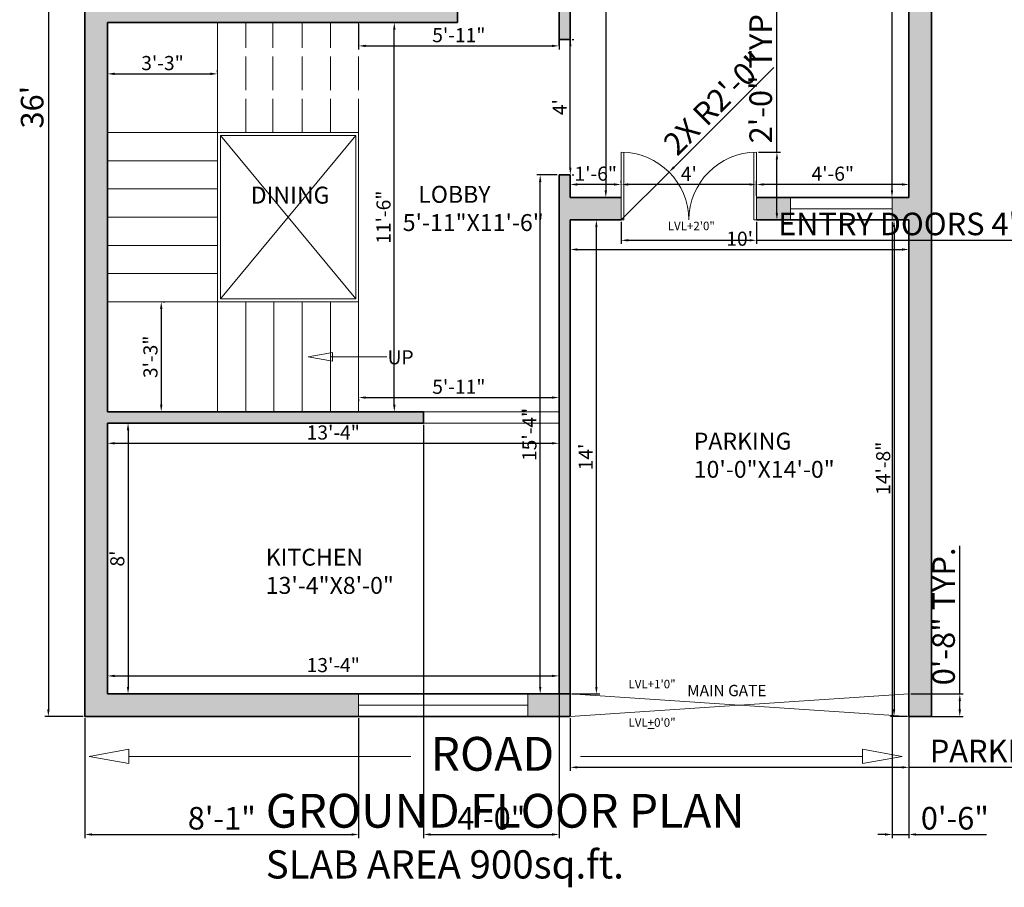
# Model space of a CAD drawing. Units: inches. Extents: x 3259 to 4981, y 1402 to 2026.
# Tile 8 of 11: x 4265 to 4614, y 1415 to 1722. Entities that reach past the tile are written whole.
import ezdxf

# ---------------------------------------------------------------- set-up
doc = ezdxf.new("R2010")
doc.units = ezdxf.units.IN
doc.linetypes.add('ACAD_ISO02W100', pattern=[15, 12, -3])
for name, color, linetype, lineweight in [('A-ANNO-DIMS', 2, 'Continuous', 13), ('A-ANNO-SYMB', 7, 'Continuous', 13), ('A-ANNO-TEXT', 7, 'Continuous', 18), ('A-ANNO-TITL', 7, 'Continuous', 25), ('A-AREA-IDEN', 7, 'Continuous', 18), ('A-DOOR', 3, 'Continuous', 18), ('A-FLOR-STRS', 7, 'Continuous', 18), ('A-FLOR-STRS-OVHD', 8, 'ACAD_ISO02W100', 13), ('A-FURN', 8, 'Continuous', 13), ('A-GLAZ', 4, 'Continuous', 18), ('A-WALL', 7, 'Continuous', 35), ('A-WALL-PATT', 252, 'Continuous', 13)]:
    doc.layers.add(name, color=color, linetype=linetype, lineweight=lineweight)
doc.styles.get("Standard").update_dxf_attribs({"font": 'arial.ttf'})
doc.dimstyles.new('ISO-25', dxfattribs={"dimtxt": 8, "dimasz": 2.5, "dimexe": 1.25, "dimexo": 0.625, "dimtad": 1, "dimdec": 1, "dimlunit": 3, "dimtxsty": 'Standard', "dimcen": 2.5, "dimclrd": 4, "dimclre": 4, "dimclrt": 1, "dimadec": 0, "dimazin": 0, "dimtfac": 1, "dimtdec": 1, "dimtmove": 0, "dimatfit": 3, "dimfxl": 1, "dimarcsym": 0})

# ---------------------------------------------------------------- blocks, each defined once
blk = doc.blocks.new('*D84')
at = {"layer": 'A-ANNO-DIMS', "color": 0, "lineweight": -2, "transparency": 16777216}
for p, q in [((4287.71, 1907.12), (4274.14, 1907.12)), ((4275.39, 1904.62), (4275.39, 1477.62)), ((4287.71, 1475.12), (4274.14, 1475.12))]:
    blk.add_line(p, q, dxfattribs=at)
at = {"layer": 'A-ANNO-DIMS', "color": 0, "transparency": 16777216}
for points in [[(4274.97, 1904.62), (4275.81, 1904.62), (4275.39, 1907.12)], [(4274.97, 1477.62), (4275.81, 1477.62), (4275.39, 1475.12)]]:
    blk.add_solid(points, dxfattribs=at)
at = {"layer": 'Defpoints', "color": 0, "transparency": 16777216}
for p in [(4288.33, 1907.12), (4275.39, 1475.12), (4288.33, 1475.12)]:
    blk.add_point(p, dxfattribs=at)
at = {"layer": 'A-ANNO-DIMS', "color": 0, "transparency": 16777216, "insert": (4270.68, 1691.12), "char_height": 8, "attachment_point": 5, "rotation": 90}
blk.add_mtext("36'", dxfattribs=at)
blk = doc.blocks.new('*D80')
at = {"layer": 'A-ANNO-DIMS', "color": 0, "lineweight": -2, "transparency": 16777216}
for p, q in [((4460.96, 1847.12), (4474.15, 1847.12)), ((4472.9, 1844.62), (4472.9, 1661.62)), ((4460.96, 1659.12), (4474.15, 1659.12))]:
    blk.add_line(p, q, dxfattribs=at)
at = {"layer": 'A-ANNO-DIMS', "color": 0, "transparency": 16777216}
for points in [[(4472.49, 1844.62), (4473.32, 1844.62), (4472.9, 1847.12)], [(4472.49, 1661.62), (4473.32, 1661.62), (4472.9, 1659.12)]]:
    blk.add_solid(points, dxfattribs=at)
at = {"layer": 'Defpoints', "color": 0, "transparency": 16777216}
for p in [(4460.33, 1847.12), (4460.33, 1659.12), (4472.9, 1659.12)]:
    blk.add_point(p, dxfattribs=at)
at = {"layer": 'A-ANNO-DIMS', "color": 0, "transparency": 16777216, "insert": (4469.73, 1753.12), "char_height": 5, "attachment_point": 5, "rotation": 90}
blk.add_mtext('15\'-8"', dxfattribs=at)
blk = doc.blocks.new('*D81')
at = {"layer": 'A-ANNO-DIMS', "color": 0, "lineweight": -2, "transparency": 16777216}
for p, q in [((4385.33, 1587.56), (4385.33, 1586.93)), ((4387.83, 1588.18), (4453.83, 1588.18)), ((4456.33, 1588.81), (4456.33, 1589.43))]:
    blk.add_line(p, q, dxfattribs=at)
at = {"layer": 'A-ANNO-DIMS', "color": 0, "transparency": 16777216}
for points in [[(4387.83, 1588.6), (4387.83, 1587.76), (4385.33, 1588.18)], [(4453.83, 1588.6), (4453.83, 1587.76), (4456.33, 1588.18)]]:
    blk.add_solid(points, dxfattribs=at)
at = {"layer": 'Defpoints', "color": 0, "transparency": 16777216}
for p in [(4385.33, 1588.18), (4456.33, 1588.18), (4456.33, 1588.18)]:
    blk.add_point(p, dxfattribs=at)
at = {"layer": 'A-ANNO-DIMS', "color": 0, "transparency": 16777216, "insert": (4420.83, 1591.36), "char_height": 5, "attachment_point": 5}
blk.add_mtext('5\'-11"', dxfattribs=at)
blk = doc.blocks.new('*D82')
at = {"layer": 'A-ANNO-DIMS', "color": 0, "lineweight": -2, "transparency": 16777216}
for p, q in [((4396.19, 1721.12), (4399.22, 1721.12)), ((4397.97, 1585.62), (4397.97, 1718.62)), ((4393.89, 1583.12), (4399.22, 1583.12))]:
    blk.add_line(p, q, dxfattribs=at)
at = {"layer": 'A-ANNO-DIMS', "color": 0, "transparency": 16777216}
for points in [[(4397.55, 1718.62), (4398.39, 1718.62), (4397.97, 1721.12)], [(4397.55, 1585.62), (4398.39, 1585.62), (4397.97, 1583.12)]]:
    blk.add_solid(points, dxfattribs=at)
at = {"layer": 'Defpoints', "color": 0, "transparency": 16777216}
for p in [(4395.56, 1721.12), (4397.97, 1721.12), (4393.26, 1583.12)]:
    blk.add_point(p, dxfattribs=at)
at = {"layer": 'A-ANNO-DIMS', "color": 0, "transparency": 16777216, "insert": (4394.79, 1652.12), "char_height": 5, "attachment_point": 5, "rotation": 90}
blk.add_mtext('11\'-6"', dxfattribs=at)
blk = doc.blocks.new('*D74')
at = {"layer": 'A-ANNO-DIMS', "color": 0, "lineweight": -2, "transparency": 16777216}
for p, q in [((4296.33, 1703.55), (4296.33, 1704.17)), ((4298.83, 1702.92), (4332.83, 1702.92)), ((4335.33, 1703.55), (4335.33, 1704.17))]:
    blk.add_line(p, q, dxfattribs=at)
at = {"layer": 'A-ANNO-DIMS', "color": 0, "transparency": 16777216}
for points in [[(4298.83, 1703.34), (4298.83, 1702.51), (4296.33, 1702.92)], [(4332.83, 1703.34), (4332.83, 1702.51), (4335.33, 1702.92)]]:
    blk.add_solid(points, dxfattribs=at)
at = {"layer": 'Defpoints', "color": 0, "transparency": 16777216}
for p in [(4296.33, 1702.92), (4335.33, 1702.92), (4335.33, 1702.92)]:
    blk.add_point(p, dxfattribs=at)
at = {"layer": 'A-ANNO-DIMS', "color": 0, "transparency": 16777216, "insert": (4315.83, 1706.1), "char_height": 5, "attachment_point": 5}
blk.add_mtext('3\'-3"', dxfattribs=at)
blk = doc.blocks.new('*D75')
at = {"layer": 'A-ANNO-DIMS', "color": 0, "lineweight": -2, "transparency": 16777216}
for p, q in [((4315.38, 1619.62), (4315.38, 1585.62)), ((4316.01, 1622.12), (4316.63, 1622.12)), ((4316.01, 1583.12), (4316.63, 1583.12))]:
    blk.add_line(p, q, dxfattribs=at)
at = {"layer": 'A-ANNO-DIMS', "color": 0, "transparency": 16777216}
for points in [[(4314.97, 1619.62), (4315.8, 1619.62), (4315.38, 1622.12)], [(4314.97, 1585.62), (4315.8, 1585.62), (4315.38, 1583.12)]]:
    blk.add_solid(points, dxfattribs=at)
at = {"layer": 'Defpoints', "color": 0, "transparency": 16777216}
for p in [(4315.38, 1622.12), (4315.38, 1583.12), (4315.38, 1583.12)]:
    blk.add_point(p, dxfattribs=at)
at = {"layer": 'A-ANNO-DIMS', "color": 0, "transparency": 16777216, "insert": (4312.2, 1602.62), "char_height": 5, "attachment_point": 5, "rotation": 90}
blk.add_mtext('3\'-3"', dxfattribs=at)
blk = doc.blocks.new('*D76')
at = {"layer": 'A-ANNO-DIMS', "color": 0, "lineweight": -2, "transparency": 16777216}
for p, q in [((4296.33, 1578.49), (4296.33, 1570.72)), ((4456.33, 1578.49), (4456.33, 1570.72)), ((4298.83, 1571.97), (4453.83, 1571.97))]:
    blk.add_line(p, q, dxfattribs=at)
at = {"layer": 'A-ANNO-DIMS', "color": 0, "transparency": 16777216}
for points in [[(4298.83, 1572.39), (4298.83, 1571.56), (4296.33, 1571.97)], [(4453.83, 1572.39), (4453.83, 1571.56), (4456.33, 1571.97)]]:
    blk.add_solid(points, dxfattribs=at)
at = {"layer": 'Defpoints', "color": 0, "transparency": 16777216}
for p in [(4296.33, 1579.12), (4456.33, 1579.12), (4456.33, 1571.97)]:
    blk.add_point(p, dxfattribs=at)
at = {"layer": 'A-ANNO-DIMS', "color": 0, "transparency": 16777216, "insert": (4376.33, 1575.15), "char_height": 5, "attachment_point": 5}
blk.add_mtext('13\'-4"', dxfattribs=at)
blk = doc.blocks.new('*D77')
at = {"layer": 'A-ANNO-DIMS', "color": 0, "lineweight": -2, "transparency": 16777216}
for p, q in [((4296.96, 1579.12), (4304.87, 1579.12)), ((4303.62, 1576.62), (4303.62, 1485.62)), ((4296.96, 1483.12), (4304.87, 1483.12))]:
    blk.add_line(p, q, dxfattribs=at)
at = {"layer": 'A-ANNO-DIMS', "color": 0, "transparency": 16777216}
for points in [[(4303.21, 1576.62), (4304.04, 1576.62), (4303.62, 1579.12)], [(4303.21, 1485.62), (4304.04, 1485.62), (4303.62, 1483.12)]]:
    blk.add_solid(points, dxfattribs=at)
at = {"layer": 'Defpoints', "color": 0, "transparency": 16777216}
for p in [(4296.33, 1579.12), (4296.33, 1483.12), (4303.62, 1483.12)]:
    blk.add_point(p, dxfattribs=at)
at = {"layer": 'A-ANNO-DIMS', "color": 0, "transparency": 16777216, "insert": (4300.45, 1531.12), "char_height": 5, "attachment_point": 5, "rotation": 90}
blk.add_mtext("8'", dxfattribs=at)
blk = doc.blocks.new('*D78')
at = {"layer": 'A-ANNO-DIMS', "color": 0, "lineweight": -2, "transparency": 16777216}
for p, q in [((4460.96, 1651.12), (4470.82, 1651.12)), ((4469.57, 1485.62), (4469.57, 1648.62)), ((4460.96, 1483.12), (4470.82, 1483.12))]:
    blk.add_line(p, q, dxfattribs=at)
at = {"layer": 'A-ANNO-DIMS', "color": 0, "transparency": 16777216}
for points in [[(4469.16, 1648.62), (4469.99, 1648.62), (4469.57, 1651.12)], [(4469.16, 1485.62), (4469.99, 1485.62), (4469.57, 1483.12)]]:
    blk.add_solid(points, dxfattribs=at)
at = {"layer": 'Defpoints', "color": 0, "transparency": 16777216}
for p in [(4460.33, 1651.12), (4469.57, 1651.12), (4460.33, 1483.12)]:
    blk.add_point(p, dxfattribs=at)
at = {"layer": 'A-ANNO-DIMS', "color": 0, "transparency": 16777216, "insert": (4466.44, 1567.12), "char_height": 5, "attachment_point": 5, "rotation": 90}
blk.add_mtext("14'", dxfattribs=at)
blk = doc.blocks.new('*D64')
at = {"layer": 'A-ANNO-DIMS', "color": 0, "lineweight": -2, "transparency": 16777216}
for p, q in [((4460.33, 1650.49), (4460.33, 1639.41)), ((4580.33, 1650.49), (4580.33, 1639.41)), ((4462.83, 1640.66), (4577.83, 1640.66))]:
    blk.add_line(p, q, dxfattribs=at)
at = {"layer": 'A-ANNO-DIMS', "color": 0, "transparency": 16777216}
for points in [[(4462.83, 1641.08), (4462.83, 1640.25), (4460.33, 1640.66)], [(4577.83, 1641.08), (4577.83, 1640.25), (4580.33, 1640.66)]]:
    blk.add_solid(points, dxfattribs=at)
at = {"layer": 'Defpoints', "color": 0, "transparency": 16777216}
for p in [(4460.33, 1651.12), (4580.33, 1651.12), (4580.33, 1640.66)]:
    blk.add_point(p, dxfattribs=at)
at = {"layer": 'A-ANNO-DIMS', "color": 0, "transparency": 16777216, "insert": (4520.33, 1643.84), "char_height": 5, "attachment_point": 5}
blk.add_mtext("10'", dxfattribs=at)
blk = doc.blocks.new('*D107')
at = {"layer": 'A-ANNO-DIMS', "color": 0, "lineweight": -2, "transparency": 16777216}
for p, q in [((4296.33, 1483.74), (4296.33, 1490.78)), ((4456.33, 1483.74), (4456.33, 1490.78)), ((4298.83, 1489.53), (4453.83, 1489.53))]:
    blk.add_line(p, q, dxfattribs=at)
at = {"layer": 'A-ANNO-DIMS', "color": 0, "transparency": 16777216}
for points in [[(4298.83, 1489.94), (4298.83, 1489.11), (4296.33, 1489.53)], [(4453.83, 1489.94), (4453.83, 1489.11), (4456.33, 1489.53)]]:
    blk.add_solid(points, dxfattribs=at)
at = {"layer": 'Defpoints', "color": 0, "transparency": 16777216}
for p in [(4456.33, 1489.53), (4296.33, 1483.12), (4456.33, 1483.12)]:
    blk.add_point(p, dxfattribs=at)
at = {"layer": 'A-ANNO-DIMS', "color": 0, "transparency": 16777216, "insert": (4376.33, 1492.71), "char_height": 5, "attachment_point": 5}
blk.add_mtext('13\'-4"', dxfattribs=at)
blk = doc.blocks.new('*D108')
at = {"layer": 'A-ANNO-DIMS', "color": 0, "lineweight": -2, "transparency": 16777216}
for p, q in [((4455.71, 1667.12), (4448.41, 1667.12)), ((4449.66, 1485.62), (4449.66, 1664.62)), ((4455.71, 1483.12), (4448.41, 1483.12))]:
    blk.add_line(p, q, dxfattribs=at)
at = {"layer": 'A-ANNO-DIMS', "color": 0, "transparency": 16777216}
for points in [[(4449.24, 1664.62), (4450.08, 1664.62), (4449.66, 1667.12)], [(4449.24, 1485.62), (4450.08, 1485.62), (4449.66, 1483.12)]]:
    blk.add_solid(points, dxfattribs=at)
at = {"layer": 'Defpoints', "color": 0, "transparency": 16777216}
for p in [(4449.66, 1667.12), (4456.33, 1667.12), (4456.33, 1483.12)]:
    blk.add_point(p, dxfattribs=at)
at = {"layer": 'A-ANNO-DIMS', "color": 0, "transparency": 16777216, "insert": (4446.48, 1575.12), "char_height": 5, "attachment_point": 5, "rotation": 90}
blk.add_mtext('15\'-4"', dxfattribs=at)
blk = doc.blocks.new('*D115')
at = {"layer": 'A-ANNO-DIMS', "color": 0, "lineweight": -2, "transparency": 16777216}
for p, q in [((4579.71, 1851.12), (4573.06, 1851.12)), ((4574.31, 1848.62), (4574.31, 1661.62)), ((4579.71, 1659.12), (4573.06, 1659.12))]:
    blk.add_line(p, q, dxfattribs=at)
at = {"layer": 'A-ANNO-DIMS', "color": 0, "transparency": 16777216}
for points in [[(4573.9, 1848.62), (4574.73, 1848.62), (4574.31, 1851.12)], [(4573.9, 1661.62), (4574.73, 1661.62), (4574.31, 1659.12)]]:
    blk.add_solid(points, dxfattribs=at)
at = {"layer": 'Defpoints', "color": 0, "transparency": 16777216}
for p in [(4580.33, 1851.12), (4574.31, 1659.12), (4580.33, 1659.12)]:
    blk.add_point(p, dxfattribs=at)
at = {"layer": 'A-ANNO-DIMS', "color": 0, "transparency": 16777216, "insert": (4571.13, 1755.12), "char_height": 5, "attachment_point": 5, "rotation": 90}
blk.add_mtext("16'", dxfattribs=at)
blk = doc.blocks.new('*D116')
at = {"layer": 'A-ANNO-DIMS', "color": 0, "lineweight": -2, "transparency": 16777216}
for p, q in [((4526.33, 1659.74), (4526.33, 1664.96)), ((4580.33, 1659.74), (4580.33, 1664.96)), ((4577.83, 1663.71), (4528.83, 1663.71))]:
    blk.add_line(p, q, dxfattribs=at)
at = {"layer": 'A-ANNO-DIMS', "color": 0, "transparency": 16777216}
for points in [[(4528.83, 1664.13), (4528.83, 1663.29), (4526.33, 1663.71)], [(4577.83, 1664.13), (4577.83, 1663.29), (4580.33, 1663.71)]]:
    blk.add_solid(points, dxfattribs=at)
at = {"layer": 'Defpoints', "color": 0, "transparency": 16777216}
for p in [(4526.33, 1663.71), (4526.33, 1659.12), (4580.33, 1659.12)]:
    blk.add_point(p, dxfattribs=at)
at = {"layer": 'A-ANNO-DIMS', "color": 0, "transparency": 16777216, "insert": (4553.33, 1666.89), "char_height": 5, "attachment_point": 5}
blk.add_mtext('4\'-6"', dxfattribs=at)
blk = doc.blocks.new('*D117')
at = {"layer": 'A-ANNO-DIMS', "color": 0, "lineweight": -2, "transparency": 16777216}
for p, q in [((4478.33, 1664.34), (4478.33, 1664.96)), ((4526.33, 1659.74), (4526.33, 1664.96)), ((4523.83, 1663.71), (4480.83, 1663.71))]:
    blk.add_line(p, q, dxfattribs=at)
at = {"layer": 'A-ANNO-DIMS', "color": 0, "transparency": 16777216}
for points in [[(4480.83, 1664.13), (4480.83, 1663.29), (4478.33, 1663.71)], [(4523.83, 1664.13), (4523.83, 1663.29), (4526.33, 1663.71)]]:
    blk.add_solid(points, dxfattribs=at)
at = {"layer": 'Defpoints', "color": 0, "transparency": 16777216}
for p in [(4478.33, 1663.71), (4478.33, 1663.71), (4526.33, 1659.12)]:
    blk.add_point(p, dxfattribs=at)
at = {"layer": 'A-ANNO-DIMS', "color": 0, "transparency": 16777216, "insert": (4502.33, 1666.84), "char_height": 5, "attachment_point": 5}
blk.add_mtext("4'", dxfattribs=at)
blk = doc.blocks.new('*D118')
at = {"layer": 'A-ANNO-DIMS', "color": 0, "lineweight": -2, "transparency": 16777216}
for p, q in [((4460.33, 1663.74), (4460.33, 1664.96)), ((4478.33, 1664.34), (4478.33, 1664.96)), ((4475.83, 1663.71), (4462.83, 1663.71))]:
    blk.add_line(p, q, dxfattribs=at)
at = {"layer": 'A-ANNO-DIMS', "color": 0, "transparency": 16777216}
for points in [[(4462.83, 1664.13), (4462.83, 1663.29), (4460.33, 1663.71)], [(4475.83, 1664.13), (4475.83, 1663.29), (4478.33, 1663.71)]]:
    blk.add_solid(points, dxfattribs=at)
at = {"layer": 'Defpoints', "color": 0, "transparency": 16777216}
for p in [(4460.33, 1663.71), (4460.33, 1663.12), (4478.33, 1663.71)]:
    blk.add_point(p, dxfattribs=at)
at = {"layer": 'A-ANNO-DIMS', "color": 0, "transparency": 16777216, "insert": (4469.33, 1666.89), "char_height": 5, "attachment_point": 5}
blk.add_mtext('1\'-6"', dxfattribs=at)
blk = doc.blocks.new('*D119')
at = {"layer": 'A-ANNO-DIMS', "color": 0, "lineweight": -2, "transparency": 16777216}
for p, q in [((4385.33, 1720.49), (4385.33, 1711.58)), ((4456.33, 1720.49), (4456.33, 1711.58)), ((4387.83, 1712.83), (4453.83, 1712.83))]:
    blk.add_line(p, q, dxfattribs=at)
at = {"layer": 'A-ANNO-DIMS', "color": 0, "transparency": 16777216}
for points in [[(4387.83, 1713.24), (4387.83, 1712.41), (4385.33, 1712.83)], [(4453.83, 1713.24), (4453.83, 1712.41), (4456.33, 1712.83)]]:
    blk.add_solid(points, dxfattribs=at)
at = {"layer": 'Defpoints', "color": 0, "transparency": 16777216}
for p in [(4385.33, 1721.12), (4456.33, 1721.12), (4456.33, 1712.83)]:
    blk.add_point(p, dxfattribs=at)
at = {"layer": 'A-ANNO-DIMS', "color": 0, "transparency": 16777216, "insert": (4420.83, 1716), "char_height": 5, "attachment_point": 5}
blk.add_mtext('5\'-11"', dxfattribs=at)
blk = doc.blocks.new('*D120')
at = {"layer": 'A-ANNO-DIMS', "color": 0, "lineweight": -2, "transparency": 16777216}
for p, q in [((4460.96, 1715.12), (4461.58, 1715.12)), ((4460.33, 1669.62), (4460.33, 1712.62)), ((4460.96, 1667.12), (4461.58, 1667.12))]:
    blk.add_line(p, q, dxfattribs=at)
at = {"layer": 'A-ANNO-DIMS', "color": 0, "transparency": 16777216}
for points in [[(4459.91, 1712.62), (4460.75, 1712.62), (4460.33, 1715.12)], [(4459.91, 1669.62), (4460.75, 1669.62), (4460.33, 1667.12)]]:
    blk.add_solid(points, dxfattribs=at)
at = {"layer": 'Defpoints', "color": 0, "transparency": 16777216}
for p in [(4460.33, 1715.12), (4460.33, 1715.12), (4460.33, 1667.12)]:
    blk.add_point(p, dxfattribs=at)
at = {"layer": 'A-ANNO-DIMS', "color": 0, "transparency": 16777216, "insert": (4457.21, 1691.12), "char_height": 5, "attachment_point": 5, "rotation": 90}
blk.add_mtext("4'", dxfattribs=at)
blk = doc.blocks.new('*D132')
at = {"layer": 'A-ANNO-DIMS', "color": 0, "lineweight": -2, "transparency": 16777216}
for p, q in [((4579.71, 1651.12), (4573.77, 1651.12)), ((4575.02, 1648.62), (4575.02, 1477.62)), ((4579.71, 1475.12), (4573.77, 1475.12))]:
    blk.add_line(p, q, dxfattribs=at)
at = {"layer": 'A-ANNO-DIMS', "color": 0, "transparency": 16777216}
for points in [[(4574.61, 1648.62), (4575.44, 1648.62), (4575.02, 1651.12)], [(4574.61, 1477.62), (4575.44, 1477.62), (4575.02, 1475.12)]]:
    blk.add_solid(points, dxfattribs=at)
at = {"layer": 'Defpoints', "color": 0, "transparency": 16777216}
for p in [(4580.33, 1651.12), (4575.02, 1475.12), (4580.33, 1475.12)]:
    blk.add_point(p, dxfattribs=at)
at = {"layer": 'A-ANNO-DIMS', "color": 0, "transparency": 16777216, "insert": (4571.84, 1563.12), "char_height": 5, "attachment_point": 5, "rotation": 90}
blk.add_mtext('14\'-8"', dxfattribs=at)
blk = doc.blocks.new('ENTRY-DOOR-PAIR-48IN')
for p, q in [((0, 0), (0, 24)), ((1, 0), (1, 24)), ((47, 0), (47, 24)), ((48, 0), (48, 24)), ((0, 0), (0, 8)), ((48, 0), (48, 8)), ((0, 0), (1, 0)), ((48, 0), (47, 0))]:
    blk.add_line(p, q)
for centre, start, end in [((0, 0), 0, 90), ((48, 0), 90, 180)]:
    blk.add_arc(centre, 24, start, end)
blk = doc.blocks.new('PARKING-GATE-120IN')
for p, q in [((0, 8), (120, 0)), ((120, 8), (0, 0))]:
    blk.add_line(p, q)
blk = doc.blocks.new('WINDOW-60x8')
for p, q in [((0, 0), (0, 8)), ((60, 0), (60, 8)), ((0, 4), (60, 4))]:
    blk.add_line(p, q)
blk = doc.blocks.new('WINDOW-36x8')
for p, q in [((0, 0), (0, 8)), ((36, 0), (36, 8)), ((0, 4), (36, 4))]:
    blk.add_line(p, q)
blk = doc.blocks.new('STAIR-WELL-50x60')
for p, q in [((1, 59), (49, 1)), ((1, 1), (49, 59))]:
    blk.add_line(p, q)
for points in [[(50, 60), (0, 60), (0, 0), (50, 0)], [(49, 59), (1, 59), (1, 1), (49, 1)]]:
    blk.add_lwpolyline(points, close=True)
blk = doc.blocks.new('STAIR-DIRECTION')
blk.add_line((7.93, 1.55), (27.85, 1.55))
blk.add_lwpolyline([(0, 1.55), (8.64, 3.11), (8.64, 0)], close=True)
blk = doc.blocks.new('ROAD-DIRECTION')
blk.add_line((99.82, 2.55), (0, 2.55))
blk.add_lwpolyline([(113.98, 2.55), (99.82, 5.11), (99.82, 0)], close=True)
blk = doc.blocks.new('*D170')
at = {"layer": 'A-ANNO-DIMS', "color": 4, "lineweight": -2, "transparency": 16777216}
for p, q in [((4478.33, 1650.49), (4478.33, 1642.67)), ((4526.33, 1650.49), (4526.33, 1642.67)), ((4480.83, 1643.92), (4523.83, 1643.92)), ((4526.33, 1643.92), (4663.49, 1643.92))]:
    blk.add_line(p, q, dxfattribs=at)
at = {"layer": 'A-ANNO-DIMS', "color": 4, "transparency": 16777216}
for points in [[(4480.83, 1644.33), (4480.83, 1643.5), (4478.33, 1643.92)], [(4523.83, 1644.33), (4523.83, 1643.5), (4526.33, 1643.92)]]:
    blk.add_solid(points, dxfattribs=at)
at = {"layer": 'Defpoints', "color": 0, "transparency": 16777216}
for p in [(4478.33, 1651.12), (4526.33, 1651.12), (4526.33, 1643.92)]:
    blk.add_point(p, dxfattribs=at)
at = {"layer": 'A-ANNO-DIMS', "color": 1, "transparency": 16777216, "insert": (4596.16, 1648.68), "char_height": 8, "attachment_point": 5}
blk.add_mtext('ENTRY DOORS 4\'-0" TYP.', dxfattribs=at)
blk = doc.blocks.new('*D171')
at = {"layer": 'A-ANNO-DIMS', "color": 4, "lineweight": -2, "transparency": 16777216}
for p, q in [((4533.53, 1675.12), (4533.53, 1727.77)), ((4526.96, 1675.12), (4534.78, 1675.12)), ((4533.53, 1653.62), (4533.53, 1672.62)), ((4526.96, 1651.12), (4534.78, 1651.12))]:
    blk.add_line(p, q, dxfattribs=at)
at = {"layer": 'A-ANNO-DIMS', "color": 4, "transparency": 16777216}
for points in [[(4533.11, 1672.62), (4533.95, 1672.62), (4533.53, 1675.12)], [(4533.11, 1653.62), (4533.95, 1653.62), (4533.53, 1651.12)]]:
    blk.add_solid(points, dxfattribs=at)
at = {"layer": 'Defpoints', "color": 0, "transparency": 16777216}
for p in [(4526.33, 1675.12), (4533.53, 1675.12), (4526.33, 1651.12)]:
    blk.add_point(p, dxfattribs=at)
at = {"layer": 'A-ANNO-DIMS', "color": 1, "transparency": 16777216, "insert": (4528.82, 1702.69), "char_height": 8, "attachment_point": 5, "rotation": 90}
blk.add_mtext('2\'-0" TYP.', dxfattribs=at)
blk = doc.blocks.new('*D172')
at = {"layer": 'A-ANNO-DIMS', "color": 4, "lineweight": -2, "transparency": 16777216}
for p, q in [((4460.33, 1474.49), (4460.33, 1455.87)), ((4580.33, 1474.49), (4580.33, 1455.87)), ((4462.83, 1457.12), (4577.83, 1457.12)), ((4580.33, 1457.12), (4725.6, 1457.12))]:
    blk.add_line(p, q, dxfattribs=at)
at = {"layer": 'A-ANNO-DIMS', "color": 4, "transparency": 16777216}
for points in [[(4462.83, 1457.53), (4462.83, 1456.7), (4460.33, 1457.12)], [(4577.83, 1457.53), (4577.83, 1456.7), (4580.33, 1457.12)]]:
    blk.add_solid(points, dxfattribs=at)
at = {"layer": 'Defpoints', "color": 0, "transparency": 16777216}
for p in [(4460.33, 1475.12), (4580.33, 1475.12), (4580.33, 1457.12)]:
    blk.add_point(p, dxfattribs=at)
at = {"layer": 'A-ANNO-DIMS', "color": 1, "transparency": 16777216, "insert": (4654.22, 1461.88), "char_height": 8, "attachment_point": 5}
blk.add_mtext('PARKING GATE 10\'-0" TYP.', dxfattribs=at)
blk = doc.blocks.new('*D173')
at = {"layer": 'A-ANNO-DIMS', "color": 4, "lineweight": -2, "transparency": 16777216}
for p, q in [((4598.33, 1483.12), (4598.33, 1535.63)), ((4580.96, 1483.12), (4599.58, 1483.12)), ((4598.33, 1477.62), (4598.33, 1480.62)), ((4580.96, 1475.12), (4599.58, 1475.12))]:
    blk.add_line(p, q, dxfattribs=at)
at = {"layer": 'A-ANNO-DIMS', "color": 4, "transparency": 16777216}
for points in [[(4597.91, 1480.62), (4598.75, 1480.62), (4598.33, 1483.12)], [(4597.91, 1477.62), (4598.75, 1477.62), (4598.33, 1475.12)]]:
    blk.add_solid(points, dxfattribs=at)
at = {"layer": 'Defpoints', "color": 0, "transparency": 16777216}
for p in [(4580.33, 1483.12), (4598.33, 1483.12), (4580.33, 1475.12)]:
    blk.add_point(p, dxfattribs=at)
at = {"layer": 'A-ANNO-DIMS', "color": 1, "transparency": 16777216, "insert": (4593.62, 1510.62), "char_height": 8, "attachment_point": 5, "rotation": 90}
blk.add_mtext('0\'-8" TYP.', dxfattribs=at)
blk = doc.blocks.new('*D192')
at = {"layer": 'A-ANNO-DIMS', "color": 4, "lineweight": -2, "transparency": 16777216}
for p, q in [((4288.33, 1474.49), (4288.33, 1432.07)), ((4385.33, 1474.49), (4385.33, 1432.07)), ((4290.83, 1433.32), (4382.83, 1433.32))]:
    blk.add_line(p, q, dxfattribs=at)
at = {"layer": 'A-ANNO-DIMS', "color": 4, "transparency": 16777216}
for points in [[(4290.83, 1433.74), (4290.83, 1432.9), (4288.33, 1433.32)], [(4382.83, 1433.74), (4382.83, 1432.9), (4385.33, 1433.32)]]:
    blk.add_solid(points, dxfattribs=at)
at = {"layer": 'Defpoints', "color": 0, "transparency": 16777216}
for p in [(4288.33, 1475.12), (4385.33, 1475.12), (4385.33, 1433.32)]:
    blk.add_point(p, dxfattribs=at)
at = {"layer": 'A-ANNO-DIMS', "color": 1, "transparency": 16777216, "insert": (4336.83, 1438.03), "char_height": 8, "attachment_point": 5}
blk.add_mtext('8\'-1"', dxfattribs=at)
blk = doc.blocks.new('*D193')
at = {"layer": 'A-ANNO-DIMS', "color": 4, "lineweight": -2, "transparency": 16777216}
for p, q in [((4574.33, 1650.49), (4574.33, 1432.07)), ((4580.33, 1650.49), (4580.33, 1432.07)), ((4571.83, 1433.32), (4569.33, 1433.32)), ((4574.33, 1433.32), (4580.33, 1433.32)), ((4582.83, 1433.32), (4607.85, 1433.32))]:
    blk.add_line(p, q, dxfattribs=at)
at = {"layer": 'A-ANNO-DIMS', "color": 4, "transparency": 16777216}
for points in [[(4571.83, 1433.74), (4571.83, 1432.9), (4574.33, 1433.32)], [(4582.83, 1433.74), (4582.83, 1432.9), (4580.33, 1433.32)]]:
    blk.add_solid(points, dxfattribs=at)
at = {"layer": 'Defpoints', "color": 0, "transparency": 16777216}
for p in [(4574.33, 1651.12), (4580.33, 1651.12), (4580.33, 1433.32)]:
    blk.add_point(p, dxfattribs=at)
at = {"layer": 'A-ANNO-DIMS', "color": 1, "transparency": 16777216, "insert": (4596.59, 1438.03), "char_height": 8, "attachment_point": 5}
blk.add_mtext('0\'-6"', dxfattribs=at)
blk = doc.blocks.new('*D194')
at = {"layer": 'A-ANNO-DIMS', "color": 4, "lineweight": -2, "transparency": 16777216}
for p, q in [((4408.33, 1578.49), (4408.33, 1432.07)), ((4456.33, 1578.49), (4456.33, 1432.07)), ((4410.83, 1433.32), (4453.83, 1433.32))]:
    blk.add_line(p, q, dxfattribs=at)
at = {"layer": 'A-ANNO-DIMS', "color": 4, "transparency": 16777216}
for points in [[(4410.83, 1433.74), (4410.83, 1432.9), (4408.33, 1433.32)], [(4453.83, 1433.74), (4453.83, 1432.9), (4456.33, 1433.32)]]:
    blk.add_solid(points, dxfattribs=at)
at = {"layer": 'Defpoints', "color": 0, "transparency": 16777216}
for p in [(4408.33, 1579.12), (4456.33, 1579.12), (4456.33, 1433.32)]:
    blk.add_point(p, dxfattribs=at)
at = {"layer": 'A-ANNO-DIMS', "color": 1, "transparency": 16777216, "insert": (4432.33, 1438.03), "char_height": 8, "attachment_point": 5}
blk.add_mtext('4\'-0"', dxfattribs=at)
blk = doc.blocks.new('*D202')
at = {"layer": 'A-ANNO-DIMS', "color": 4, "lineweight": -2, "transparency": 16777216}
for p, q in [((4532.42, 1705.21), (4497.07, 1669.86)), ((4478.33, 1651.12), (4495.3, 1668.09))]:
    blk.add_line(p, q, dxfattribs=at)
at = {"layer": 'A-ANNO-DIMS', "color": 4, "transparency": 16777216}
blk.add_solid([(4496.77, 1670.15), (4497.36, 1669.56), (4495.3, 1668.09)], dxfattribs=at)
at = {"layer": 'Defpoints', "color": 0, "transparency": 16777216}
for p in [(4495.3, 1668.09), (4478.33, 1651.12)]:
    blk.add_point(p, dxfattribs=at)
at = {"layer": 'A-ANNO-DIMS', "color": 1, "transparency": 16777216, "insert": (4512.3, 1691.75), "char_height": 8, "attachment_point": 5, "rotation": 44.9997}
blk.add_mtext('2X R2\'-0"', dxfattribs=at)

msp = doc.modelspace()

# ---------------------------------------------------------------- hatches: boundary and pattern name
at = {"layer": 'A-WALL-PATT'}
h = msp.add_hatch(color=256, dxfattribs=at)
h.dxf.hatch_style = 1
h.paths.add_polyline_path([(4588.33, 1907.12), (4288.33, 1907.12), (4288.33, 1475.12), (4385.33, 1475.12), (4385.33, 1483.12), (4296.33, 1483.12), (4296.33, 1579.12), (4408.33, 1579.12), (4408.33, 1583.12), (4296.33, 1583.12), (4296.33, 1721.12), (4420.33, 1721.12), (4420.33, 1725.12), (4296.33, 1725.12), (4296.33, 1899.12), (4332.33, 1899.12), (4332.33, 1881.12), (4336.33, 1881.12), (4336.33, 1899.12), (4416.33, 1899.12), (4416.33, 1887.12), (4420.33, 1887.12), (4420.33, 1899.12), (4492.33, 1899.12), (4492.33, 1887.12), (4496.33, 1887.12), (4496.33, 1899.12), (4580.33, 1899.12), (4580.33, 1851.12), (4526.33, 1851.12), (4526.33, 1847.12), (4580.33, 1847.12), (4580.33, 1659.12), (4574.33, 1659.12), (4574.33, 1651.12), (4580.33, 1651.12), (4580.33, 1475.12), (4588.33, 1475.12)])
h.paths.add_polyline_path([(4420.33, 1863.12), (4416.33, 1863.12), (4416.33, 1851.12), (4332.33, 1851.12), (4332.33, 1847.12), (4370.16, 1847.12), (4370.16, 1847.13), (4370.21, 1847.13), (4370.21, 1847.12), (4374.23, 1847.12), (4374.23, 1847.12), (4374.28, 1847.12), (4420.33, 1847.12)], flags=17)
h.paths.add_polyline_path([(4496.33, 1863.12), (4492.33, 1863.12), (4492.33, 1847.12), (4496.33, 1847.12)], flags=17)
h.paths.add_polyline_path([(4460.33, 1851.12), (4456.33, 1851.12), (4456.33, 1715.12), (4460.33, 1715.12), (4460.33, 1777.43), (4460.32, 1777.43), (4460.32, 1777.47), (4460.33, 1777.47), (4460.33, 1781.5), (4460.33, 1781.5), (4460.33, 1781.55)], flags=17)
h.paths.add_polyline_path([(4478.33, 1659.12), (4460.33, 1659.12), (4460.33, 1667.12), (4456.33, 1667.12), (4456.33, 1483.12), (4460.33, 1483.12), (4460.33, 1651.12), (4478.33, 1651.12)], flags=17)
h.paths.add_polyline_path([(4538.33, 1659.12), (4526.33, 1659.12), (4526.33, 1651.12), (4538.33, 1651.12)], flags=17)
h.paths.add_polyline_path([(4460.33, 1483.12), (4445.33, 1483.12), (4445.33, 1475.12), (4460.33, 1475.12)], flags=17)

# ---------------------------------------------------------------- linework, layer by layer
at = {"layer": 'A-DOOR'}
for p, q in [((4408.33, 1583.12), (4456.33, 1583.12)), ((4408.33, 1579.12), (4456.33, 1579.12))]:
    msp.add_line(p, q, dxfattribs=at)
at = {"layer": 'A-FLOR-STRS'}
for p, q in [((4335.33, 1583.12), (4335.33, 1721.12)), ((4296.33, 1682.12), (4385.33, 1682.12)), ((4296.33, 1672.12), (4335.33, 1672.12)), ((4296.33, 1662.12), (4335.33, 1662.12)), ((4296.33, 1652.12), (4335.33, 1652.12)), ((4296.33, 1642.12), (4335.33, 1642.12)), ((4296.33, 1632.12), (4335.33, 1632.12)), ((4385.33, 1622.12), (4296.33, 1622.12)), ((4345.33, 1583.12), (4345.33, 1622.12)), ((4355.33, 1583.12), (4355.33, 1622.12)), ((4365.33, 1583.12), (4365.33, 1622.12)), ((4375.33, 1583.12), (4375.33, 1622.12)), ((4385.33, 1583.12), (4385.33, 1622.12))]:
    msp.add_line(p, q, dxfattribs=at)
at = {"layer": 'A-FLOR-STRS-OVHD'}
for p, q in [((4345.33, 1682.12), (4345.33, 1721.12)), ((4354.95, 1682.12), (4354.95, 1721.12)), ((4365.33, 1682.12), (4365.33, 1721.12)), ((4375.33, 1682.12), (4375.33, 1721.12)), ((4385.33, 1682.12), (4385.33, 1721.12))]:
    msp.add_line(p, q, dxfattribs=at)
at = {"layer": 'A-FURN'}
msp.add_line((4356.1, 1682.12), (4350.55, 1682.12), dxfattribs=at)
at = {"layer": 'A-WALL'}
for p, q in [((4456.33, 1713.12), (4456.33, 1851.12)), ((4460.33, 1713.12), (4460.33, 1851.12)), ((4580.33, 1847.12), (4580.33, 1659.12)), ((4420.33, 1721.12), (4420.33, 1725.12)), ((4296.33, 1721.12), (4420.33, 1721.12)), ((4296.33, 1583.12), (4296.33, 1721.12)), ((4456.33, 1715.12), (4460.33, 1715.12)), ((4456.33, 1483.12), (4456.33, 1667.12)), ((4456.33, 1667.12), (4460.33, 1667.12)), ((4460.33, 1659.12), (4460.33, 1667.12)), ((4460.33, 1659.12), (4478.33, 1659.12)), ((4526.33, 1659.12), (4580.33, 1659.12)), ((4460.33, 1475.12), (4460.33, 1651.12)), ((4460.33, 1651.12), (4478.33, 1651.12)), ((4526.33, 1651.12), (4580.33, 1651.12)), ((4580.33, 1651.12), (4580.33, 1475.12)), ((4408.33, 1583.12), (4296.33, 1583.12)), ((4408.33, 1579.12), (4408.33, 1583.12)), ((4296.33, 1483.12), (4296.33, 1579.12)), ((4408.33, 1579.12), (4296.33, 1579.12)), ((4460.33, 1483.12), (4296.33, 1483.12))]:
    msp.add_line(p, q, dxfattribs=at)
msp.add_lwpolyline([(4460.33, 1475.12), (4288.33, 1475.12), (4288.33, 1907.12), (4588.33, 1907.12), (4588.33, 1475.12), (4580.33, 1475.12)], dxfattribs=at)

# ---------------------------------------------------------------- block references
at = {"layer": 'A-ANNO-SYMB'}
for name, p in [('STAIR-DIRECTION', (4367.44, 1601.06)), ('ROAD-DIRECTION', (4463.98, 1458.42))]:
    msp.add_blockref(name, p, dxfattribs=at)
at = {"layer": 'A-ANNO-SYMB', "rotation": 180}
msp.add_blockref('ROAD-DIRECTION', (4403.77, 1463.53), dxfattribs=at)
at = {"layer": 'A-DOOR'}
for name, p in [('ENTRY-DOOR-PAIR-48IN', (4478.33, 1651.12)), ('PARKING-GATE-120IN', (4460.33, 1475.12))]:
    msp.add_blockref(name, p, dxfattribs=at)
at = {"layer": 'A-FLOR-STRS'}
msp.add_blockref('STAIR-WELL-50x60', (4335.33, 1622.12), dxfattribs=at)
at = {"layer": 'A-GLAZ', "rotation": 180}
msp.add_blockref('WINDOW-36x8', (4574.33, 1659.12), dxfattribs=at)
at = {"layer": 'A-GLAZ'}
msp.add_blockref('WINDOW-60x8', (4385.33, 1475.12), dxfattribs=at)

# ---------------------------------------------------------------- texts
at = {"layer": 'A-ANNO-SYMB'}
for s, width, insert, char_height, attachment_point in [('{LVL+2\'0"}', 127.3061, (4494.86, 1650.51), 3, 1), ('UP', 10.7355, (4404.81, 1604.94), 5, 3), ('{LVL+1\'0"}', 127.3061, (4480.95, 1488.13), 3, 1), ('{LVL\\L+\\l0\'0"}', 127.3061, (4480.95, 1474.51), 3, 1)]:
    msp.add_mtext_dynamic_manual_height_columns(s, width=width, gutter_width=12.5, heights=[0], dxfattribs=dict(at, insert=insert, char_height=char_height, attachment_point=attachment_point))
at = {"layer": 'A-ANNO-TEXT', "attachment_point": 1}
for s, width, insert, char_height in [('\\pxt3;MAIN GATE', 127.3061, (4501.73, 1486.34), 4), ('  ROAD', 86.9528, (4403.51, 1467.9), 12)]:
    msp.add_mtext_dynamic_manual_height_columns(s, width=width, gutter_width=12.5, heights=[0], dxfattribs=dict(at, insert=insert, char_height=char_height))
at = {"layer": 'A-ANNO-TITL', "insert": (4352.41, 1447.72), "char_height": 12, "attachment_point": 1}
msp.add_mtext_dynamic_manual_height_columns('GROUND FLOOR PLAN\\P{\\H0.83333x;SLAB AREA 900sq.ft.}', width=298.7081, gutter_width=12.5, heights=[0], dxfattribs=at)
at = {"layer": 'A-AREA-IDEN', "char_height": 6, "attachment_point": 1}
for s, insert in [('DINING', (4347.09, 1662.93)), ('   LOBBY\\P5\'-11"X11\'-6"', (4400.95, 1663.21)), ('PARKING\\P10\'-0"X14\'-0"', (4504.06, 1575.74)), ('KITCHEN\\P13\'-4"X8\'-0"', (4352.41, 1534.61))]:
    msp.add_mtext_dynamic_manual_height_columns(s, width=127.3061, gutter_width=12.5, heights=[0], dxfattribs=dict(at, insert=insert))

# ---------------------------------------------------------------- dimensions: what is measured, and where the dimension line sits
at = {"layer": 'A-ANNO-DIMS'}
for base, p1, p2, override, picture, middle in [((4275.39, 1475.12), (4288.33, 1907.12), (4288.33, 1475.12), {"dimclrd": 0, "dimclre": 0, "dimclrt": 0}, '*D84', (4270.68, 1691.12)), ((4574.31, 1659.12), (4580.33, 1851.12), (4580.33, 1659.12), {"dimtxt": 5, "dimclrd": 0, "dimclre": 0, "dimclrt": 0}, '*D115', (4571.13, 1755.12)), ((4472.9, 1659.12), (4460.33, 1847.12), (4460.33, 1659.12), {"dimtxt": 5, "dimclrd": 0, "dimclre": 0, "dimclrt": 0}, '*D80', (4469.73, 1753.12)), ((4397.97, 1721.12), (4393.26, 1583.12), (4395.56, 1721.12), {"dimtxt": 5, "dimclrd": 0, "dimclre": 0, "dimclrt": 0}, '*D82', (4394.79, 1652.12)), ((4460.33, 1715.12), (4460.33, 1667.12), (4460.33, 1715.12), {"dimtxt": 5, "dimclrd": 0, "dimclre": 0, "dimclrt": 0}, '*D120', (4457.21, 1691.12)), ((4449.66, 1667.12), (4456.33, 1483.12), (4456.33, 1667.12), {"dimtxt": 5, "dimclrd": 0, "dimclre": 0, "dimclrt": 0}, '*D108', (4446.48, 1575.12)), ((4469.57, 1651.12), (4460.33, 1483.12), (4460.33, 1651.12), {"dimtxt": 5, "dimclrd": 0, "dimclre": 0, "dimclrt": 0}, '*D78', (4466.44, 1567.12)), ((4575.02, 1475.12), (4580.33, 1651.12), (4580.33, 1475.12), {"dimtxt": 5, "dimclrd": 0, "dimclre": 0, "dimclrt": 0}, '*D132', (4571.84, 1563.12)), ((4315.38, 1583.12), (4315.38, 1622.12), (4315.38, 1583.12), {"dimtxt": 5, "dimclrd": 0, "dimclre": 0, "dimclrt": 0}, '*D75', (4312.2, 1602.62)), ((4303.62, 1483.12), (4296.33, 1579.12), (4296.33, 1483.12), {"dimtxt": 5, "dimclrd": 0, "dimclre": 0, "dimclrt": 0}, '*D77', (4300.45, 1531.12))]:
    dim = msp.add_linear_dim(base=base, p1=p1, p2=p2, angle=90, dimstyle='ISO-25', override=override, dxfattribs=at)
    dim.commit()
    dim.dimension.update_dxf_attribs({"geometry": picture, "text_midpoint": middle})
for base, p1, p2, picture, middle in [((4533.53, 1675.12), (4526.33, 1651.12), (4526.33, 1675.12), '*D171', (4528.82, 1702.69)), ((4598.33, 1483.12), (4580.33, 1475.12), (4580.33, 1483.12), '*D173', (4593.62, 1510.62))]:
    dim = msp.add_linear_dim(base=base, p1=p1, p2=p2, angle=90, text='<> TYP.', dimstyle='ISO-25', override={"dimdec": 1, "dimlfac": 1, "dimrnd": 0, "dimzin": 1, "dimdsep": 46, "dimlunit": 4, "dimfrac": 2}, dxfattribs=at)
    dim.commit()
    dim.dimension.update_dxf_attribs({"geometry": picture, "text_midpoint": middle})
for base, p1, p2, override, picture, middle in [((4456.33, 1712.83), (4385.33, 1721.12), (4456.33, 1721.12), {"dimtxt": 5, "dimclrd": 0, "dimclre": 0, "dimclrt": 0}, '*D119', (4420.83, 1716)), ((4335.33, 1702.92), (4296.33, 1702.92), (4335.33, 1702.92), {"dimtxt": 5, "dimclrd": 0, "dimclre": 0, "dimclrt": 0}, '*D74', (4315.83, 1706.1)), ((4460.33, 1663.71), (4478.33, 1663.71), (4460.33, 1663.12), {"dimtxt": 5, "dimclrd": 0, "dimclre": 0, "dimclrt": 0, "dimtmove": 1}, '*D118', (4469.33, 1666.89)), ((4478.33, 1663.71), (4526.33, 1659.12), (4478.33, 1663.71), {"dimtxt": 5, "dimclrd": 0, "dimclre": 0, "dimclrt": 0, "dimtmove": 1}, '*D117', (4502.33, 1666.84)), ((4526.33, 1663.71), (4580.33, 1659.12), (4526.33, 1659.12), {"dimtxt": 5, "dimclrd": 0, "dimclre": 0, "dimclrt": 0}, '*D116', (4553.33, 1666.89)), ((4580.33, 1640.66), (4460.33, 1651.12), (4580.33, 1651.12), {"dimtxt": 5, "dimclrd": 0, "dimclre": 0, "dimclrt": 0}, '*D64', (4520.33, 1643.84)), ((4580.33, 1433.32), (4574.33, 1651.12), (4580.33, 1651.12), {"dimdec": 1, "dimlfac": 1, "dimrnd": 0, "dimzin": 1, "dimdsep": 46, "dimlunit": 4, "dimfrac": 2}, '*D193', (4596.59, 1438.03)), ((4456.33, 1588.18), (4385.33, 1588.18), (4456.33, 1588.18), {"dimtxt": 5, "dimclrd": 0, "dimclre": 0, "dimclrt": 0}, '*D81', (4420.83, 1591.36)), ((4456.33, 1571.97), (4296.33, 1579.12), (4456.33, 1579.12), {"dimtxt": 5, "dimclrd": 0, "dimclre": 0, "dimclrt": 0}, '*D76', (4376.33, 1575.15)), ((4456.33, 1433.32), (4408.33, 1579.12), (4456.33, 1579.12), {"dimdec": 1, "dimlfac": 1, "dimrnd": 0, "dimzin": 1, "dimdsep": 46, "dimlunit": 4, "dimfrac": 2}, '*D194', (4432.33, 1438.03)), ((4456.33, 1489.53), (4296.33, 1483.12), (4456.33, 1483.12), {"dimtxt": 5, "dimclrd": 0, "dimclre": 0, "dimclrt": 0}, '*D107', (4376.33, 1492.71)), ((4385.33, 1433.32), (4288.33, 1475.12), (4385.33, 1475.12), {"dimdec": 1, "dimlfac": 1, "dimrnd": 0, "dimzin": 1, "dimdsep": 46, "dimlunit": 4, "dimfrac": 2}, '*D192', (4336.83, 1438.03))]:
    dim = msp.add_linear_dim(base=base, p1=p1, p2=p2, dimstyle='ISO-25', override=override, dxfattribs=at)
    dim.commit()
    dim.dimension.update_dxf_attribs({"geometry": picture, "text_midpoint": middle})
dim = msp.add_radius_dim(center=(4478.33, 1651.12), mpoint=(4495.3, 1668.09), text='2X <>', dimstyle='ISO-25', override={"dimdec": 1, "dimlfac": 1, "dimrnd": 0, "dimzin": 1, "dimdsep": 46, "dimlunit": 4, "dimfrac": 2}, dxfattribs=at)
dim.commit()
dim.dimension.update_dxf_attribs({"geometry": '*D202', "text_midpoint": (4512.3, 1691.75)})
for base, p1, p2, text, picture, middle in [((4526.33, 1643.92), (4478.33, 1651.12), (4526.33, 1651.12), 'ENTRY DOORS <> TYP.', '*D170', (4596.16, 1648.68)), ((4580.33, 1457.12), (4460.33, 1475.12), (4580.33, 1475.12), 'PARKING GATE <> TYP.', '*D172', (4654.22, 1461.88))]:
    dim = msp.add_linear_dim(base=base, p1=p1, p2=p2, text=text, dimstyle='ISO-25', override={"dimdec": 1, "dimlfac": 1, "dimrnd": 0, "dimzin": 1, "dimdsep": 46, "dimlunit": 4, "dimfrac": 2}, dxfattribs=at)
    dim.commit()
    dim.dimension.update_dxf_attribs({"geometry": picture, "text_midpoint": middle})

doc.saveas('drawing.dxf')
